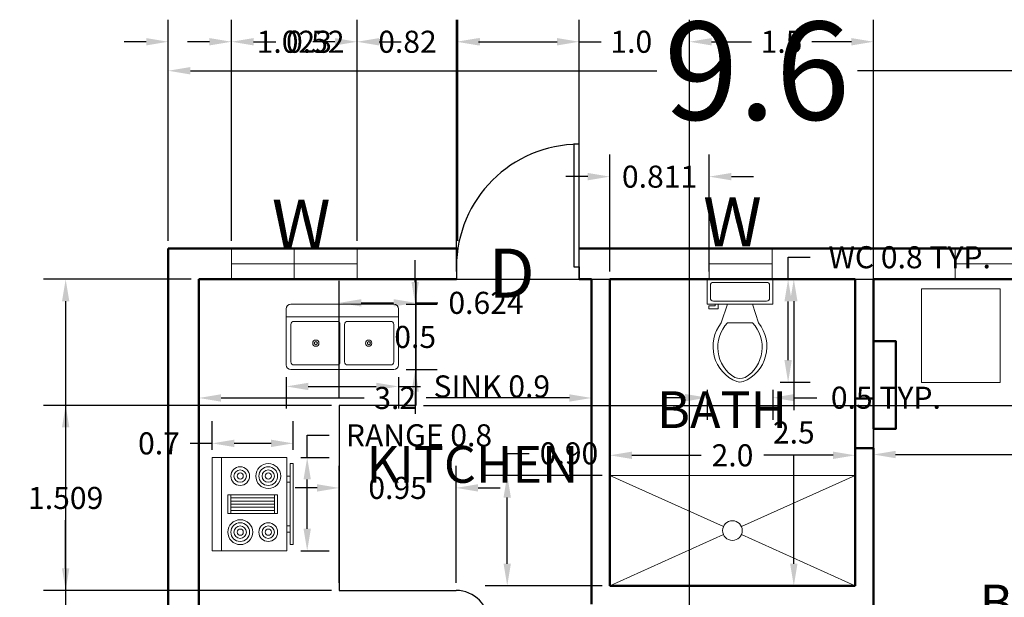
# Model space of a CAD drawing. Units: metres. Extents: x 3.9 to 21.3, y 24.8 to 56.5.
# Tile 5 of 6: x 4.9 to 13, y 36.1 to 40.8. Entities that reach past the tile are written whole.
import ezdxf

# ---------------------------------------------------------------- set-up
doc = ezdxf.new("R2010")
doc.units = ezdxf.units.M
doc.header["$MEASUREMENT"] = 0
for name, color, linetype, lineweight in [('A-AREA-IDEN', 3, 'Continuous', 25), ('A-EQPM', 6, 'Continuous', 18), ('A-FLOR-CASE', 8, 'Continuous', 25), ('A-FLOR-FIXT', 9, 'Continuous', 18), ('DIMENSIONS', 2, 'Continuous', 18), ('DOOR', 5, 'Continuous', 25), ('FURNITURE', 6, 'Continuous', 18), ('TEXT', 3, 'Continuous', 18), ('WALL', 1, 'Continuous', 50), ('WINDOW', 4, 'Continuous', 18)]:
    doc.layers.add(name, color=color, linetype=linetype, lineweight=lineweight)
doc.styles.get("Standard").update_dxf_attribs({"font": 'arial.ttf'})
doc.dimstyles.get("Standard").update_dxf_attribs({"dimtxt": 0.18, "dimasz": 0.18, "dimexe": 0.18, "dimexo": 0.0625, "dimgap": 0.09, "dimtad": 0, "dimtih": 1, "dimtoh": 1, "dimdec": 1, "dimzin": 0, "dimdsep": 46, "dimtxsty": 'Standard', "dimcen": 0.09, "dimadec": 0, "dimazin": 0, "dimtfac": 1, "dimtdec": 1, "dimtofl": 0, "dimtmove": 0, "dimatfit": 3, "dimfxl": 1, "dimtolj": 1, "dimtzin": 0, "dimarcsym": 0})

# ---------------------------------------------------------------- blocks, each defined once
blk = doc.blocks.new('*U3')
for p, q in [((0, 0), (0, -100)), ((-1000, 0), (-1000, -100))]:
    blk.add_line(p, q)
blk.add_lwpolyline([(0, 0), (0, 1000), (-43.75, 1000), (-43.75, 0)], close=True)
blk.add_arc((0, 0), 1000, 90, 180)
blk = doc.blocks.new('Range-Oven - 30 in top')
for p, q in [((0, -3), (30, -3)), ((12, -6), (18, -6)), ((13, -20), (13, -6)), ((14, -6), (14, -20)), ((15, -20), (15, -6)), ((16, -6), (16, -20)), ((17, -20), (17, -6)), ((18, -20), (12, -20)), ((6, -24), (6, -25)), ((8, -25), (8, -24)), ((22, -25), (22, -24)), ((24, -24), (24, -25))]:
    blk.add_line(p, q)
for points in [[(0, -24), (0, 0), (30, 0), (30, -24)], [(12, -21), (12, -5), (18, -5), (18, -21)], [(2, -26), (2, -25), (28, -25), (28, -26)]]:
    blk.add_lwpolyline(points, close=True)
for centre, radius in [((6, -9), 4), ((6, -9), 3), ((24, -9), 3), ((6, -9), 2), ((6, -9), 1), ((24, -9), 2), ((24, -9), 1), ((6, -18), 3), ((24, -18), 4), ((24, -18), 3), ((6, -18), 2), ((6, -18), 1), ((24, -18), 2), ((24, -18), 1)]:
    blk.add_circle(centre, radius)
blk = doc.blocks.new('Sink-double - 36 in top')
for p, q in [((-18, -4), (18, -4)), ((-0.75, -18.5), (-0.75, -6.5)), ((0.75, -6.5), (0.75, -18.5))]:
    blk.add_line(p, q)
for points in [[(-16.5, 0), (16.5, 0)], [(-18, -19.5), (-18, -1.5)], [(18, -1.5), (18, -19.5)], [(-15.5, -5.5), (-1.75, -5.5)], [(1.75, -5.5), (15.5, -5.5)], [(-16.5, -18.5), (-16.5, -6.5)], [(16.5, -6.5), (16.5, -18.5)], [(16.5, -21), (-16.5, -21)], [(-1.75, -19.5), (-15.5, -19.5)], [(15.5, -19.5), (1.75, -19.5)]]:
    blk.add_lwpolyline(points)
for centre, radius in [((-8.5, -12.5), 1), ((-8.5, -12.5), 0.5), ((8.5, -12.5), 1), ((8.5, -12.5), 0.5)]:
    blk.add_circle(centre, radius)
for centre, radius, start, end in [((-16.5, -1.5), 1.5, 90, 180), ((16.5, -1.5), 1.5, 0, 90), ((-15.5, -6.5), 1, 90, 180), ((-1.75, -6.5), 1, 0, 90), ((1.75, -6.5), 1, 90, 180), ((15.5, -6.5), 1, 0, 90), ((-15.5, -18.5), 1, 180, 270), ((-1.75, -18.5), 1, 270, 0), ((1.75, -18.5), 1, 180, 270), ((15.5, -18.5), 1, 270, 0), ((-16.5, -19.5), 1.5, 180, 270), ((16.5, -19.5), 1.5, 270, 0)]:
    blk.add_arc(centre, radius, start, end)
blk = doc.blocks.new('Toilet - top')
for p, q in [((9.5, -6), (9.5, -2)), ((-10, -8.5), (-8, -8.5)), ((-10, -9.5), (-10, -8.5)), ((-8, -8.5), (-8, -8)), ((-7, -8), (-7, -9.5)), ((-4, -8), (-6, -14)), ((4, -8), (6, -14)), ((-7, -9.5), (-10, -9.5)), ((4, -14), (-4, -14))]:
    blk.add_line(p, q)
blk.add_lwpolyline([(10.5, -8), (10.5, 0), (-10.5, 0), (-10.5, -8)], close=True)
for points in [[(-9.5, -2), (-9.5, -6)], [(8.5, -1), (-8.5, -1)], [(-8.5, -7), (8.5, -7)]]:
    blk.add_lwpolyline(points)
for centre, radius, start, end in [((-8.62, -1.88), 0.884, 81.8699, 188.1301), ((8.62, -1.88), 0.884, 351.8699, 98.1301), ((-8.62, -6.12), 0.884, 171.8699, 278.1301), ((8.62, -6.12), 0.884, 261.8699, 8.1301), ((3.52, -21.58), 12.17, 141.4691, 247.9714), ((4.2, -21.82), 11.33, 136.3677, 238.9468), ((-3.52, -21.58), 12.17, 292.0284, 38.5307), ((-4.2, -21.82), 11.33, 301.053, 43.6321), ((0, -27.88), 4, 245.7318, 294.2682), ((0, -29), 4, 254.8605, 285.1395)]:
    blk.add_arc(centre, radius, start, end)
blk = doc.blocks.new('*D22')
at = {"layer": 'Defpoints', "color": 0, "transparency": 16777216}
for p in [(15.7571, 40.3451), (6.1571, 38.8951), (15.7571, 38.8951)]:
    blk.add_point(p, dxfattribs=at)
at = {"layer": 'DIMENSIONS', "color": 0, "lineweight": -2, "transparency": 16777216}
for p, q in [((6.1571, 38.9576), (6.1571, 40.5251)), ((15.7571, 38.9576), (15.7571, 40.5251)), ((6.3371, 40.3451), (10.1392, 40.3451)), ((15.5771, 40.3451), (11.7751, 40.3451))]:
    blk.add_line(p, q, dxfattribs=at)
at = {"layer": 'DIMENSIONS', "color": 0, "transparency": 16777216}
for points in [[(6.3371, 40.3751), (6.3371, 40.3151), (6.1571, 40.3451)], [(15.5771, 40.3751), (15.5771, 40.3151), (15.7571, 40.3451)]]:
    blk.add_solid(points, dxfattribs=at)
at = {"layer": 'DIMENSIONS', "color": 0, "transparency": 16777216, "insert": (10.9571, 40.3451), "char_height": 0.18, "attachment_point": 5}
blk.add_mtext('\\A1;{\\H4.44444x;9.6}', dxfattribs=at)
blk = doc.blocks.new('*D23')
at = {"layer": 'Defpoints', "color": 0, "transparency": 16777216}
for p in [(6.4071, 37.6766), (9.6071, 37.6766), (9.6071, 37.6766)]:
    blk.add_point(p, dxfattribs=at)
at = {"layer": 'DIMENSIONS', "color": 0, "lineweight": -2, "transparency": 16777216}
for p, q in [((6.4071, 37.7391), (6.4071, 37.8566)), ((9.6071, 37.7391), (9.6071, 37.8566)), ((6.5871, 37.6766), (7.7543, 37.6766)), ((9.4271, 37.6766), (8.26, 37.6766))]:
    blk.add_line(p, q, dxfattribs=at)
at = {"layer": 'DIMENSIONS', "color": 0, "transparency": 16777216}
for points in [[(6.5871, 37.7066), (6.5871, 37.6466), (6.4071, 37.6766)], [(9.4271, 37.7066), (9.4271, 37.6466), (9.6071, 37.6766)]]:
    blk.add_solid(points, dxfattribs=at)
at = {"layer": 'DIMENSIONS', "color": 0, "transparency": 16777216, "insert": (8.0071, 37.6766), "char_height": 0.18, "attachment_point": 5}
blk.add_mtext('\\A1;3.2', dxfattribs=at)
blk = doc.blocks.new('*D24')
at = {"layer": 'Defpoints', "color": 0, "transparency": 16777216}
for p in [(9.7571, 37.2089), (11.7571, 37.2089), (11.7571, 37.2089)]:
    blk.add_point(p, dxfattribs=at)
at = {"layer": 'DIMENSIONS', "color": 0, "lineweight": -2, "transparency": 16777216}
for p, q in [((9.7571, 37.2714), (9.7571, 37.3889)), ((11.7571, 37.2714), (11.7571, 37.3889)), ((9.9371, 37.2089), (10.502, 37.2089)), ((11.5771, 37.2089), (11.0122, 37.2089))]:
    blk.add_line(p, q, dxfattribs=at)
at = {"layer": 'DIMENSIONS', "color": 0, "transparency": 16777216}
for points in [[(9.9371, 37.2389), (9.9371, 37.1789), (9.7571, 37.2089)], [(11.5771, 37.2389), (11.5771, 37.1789), (11.7571, 37.2089)]]:
    blk.add_solid(points, dxfattribs=at)
at = {"layer": 'DIMENSIONS', "color": 0, "transparency": 16777216, "insert": (10.7571, 37.2089), "char_height": 0.18, "attachment_point": 5}
blk.add_mtext('\\A1;2.0', dxfattribs=at)
blk = doc.blocks.new('*D25')
at = {"layer": 'Defpoints', "color": 0, "transparency": 16777216}
for p in [(11.9071, 37.772), (15.5071, 37.772), (15.5071, 37.2152)]:
    blk.add_point(p, dxfattribs=at)
at = {"layer": 'DIMENSIONS', "color": 0, "lineweight": -2, "transparency": 16777216}
for p, q in [((11.9071, 37.7095), (11.9071, 37.0352)), ((15.5071, 37.7095), (15.5071, 37.0352)), ((12.0871, 37.2152), (13.4534, 37.2152)), ((15.3271, 37.2152), (13.9609, 37.2152))]:
    blk.add_line(p, q, dxfattribs=at)
at = {"layer": 'DIMENSIONS', "color": 0, "transparency": 16777216}
for points in [[(12.0871, 37.2452), (12.0871, 37.1852), (11.9071, 37.2152)], [(15.3271, 37.2452), (15.3271, 37.1852), (15.5071, 37.2152)]]:
    blk.add_solid(points, dxfattribs=at)
at = {"layer": 'DIMENSIONS', "color": 0, "transparency": 16777216, "insert": (13.7071, 37.2152), "char_height": 0.18, "attachment_point": 5}
blk.add_mtext('\\A1;3.6', dxfattribs=at)
blk = doc.blocks.new('*D27')
at = {"layer": 'Defpoints', "color": 0, "transparency": 16777216}
for p in [(11.7571, 38.6451), (11.2571, 36.1451), (11.7571, 36.1451)]:
    blk.add_point(p, dxfattribs=at)
at = {"layer": 'DIMENSIONS', "color": 0, "lineweight": -2, "transparency": 16777216}
for p, q in [((11.6946, 38.6451), (11.0771, 38.6451)), ((11.2571, 38.4651), (11.2571, 37.577)), ((11.2571, 36.3251), (11.2571, 37.2132)), ((11.6946, 36.1451), (11.0771, 36.1451))]:
    blk.add_line(p, q, dxfattribs=at)
at = {"layer": 'DIMENSIONS', "color": 0, "transparency": 16777216}
for points in [[(11.2271, 38.4651), (11.2871, 38.4651), (11.2571, 38.6451)], [(11.2271, 36.3251), (11.2871, 36.3251), (11.2571, 36.1451)]]:
    blk.add_solid(points, dxfattribs=at)
at = {"layer": 'DIMENSIONS', "color": 0, "transparency": 16777216, "insert": (11.2571, 37.3951), "char_height": 0.18, "attachment_point": 5}
blk.add_mtext('\\A1;2.5', dxfattribs=at)
blk = doc.blocks.new('WIN-4-LIGHT-2046')
for p, q in [((0.5115, -0.125), (0, -0.125)), ((0.5115, -0.125), (1.0231, -0.125)), ((1.5346, -0.125), (1.0231, -0.125)), ((1.5346, -0.125), (2.0462, -0.125))]:
    blk.add_line(p, q)
for points in [[(0.5115, 0), (0, 0), (0, -0.25), (0.5115, -0.25)], [(0.5115, 0), (1.0231, 0), (1.0231, -0.25), (0.5115, -0.25)], [(1.5346, 0), (1.0231, 0), (1.0231, -0.25), (1.5346, -0.25)], [(1.5346, 0), (2.0462, 0), (2.0462, -0.25), (1.5346, -0.25)]]:
    blk.add_lwpolyline(points, close=True)
blk = doc.blocks.new('WIN-1-LIGHT-512')
blk.add_line((0, -0.125), (0.5115, -0.125))
blk.add_lwpolyline([(0, 0), (0.5115, 0), (0.5115, -0.25), (0, -0.25)], close=True)
blk = doc.blocks.new('*D45')
at = {"layer": 'Defpoints', "color": 0, "transparency": 16777216}
for p in [(11.0848, 38.6443), (11.2107, 38.6443), (11.0848, 37.8049)]:
    blk.add_point(p, dxfattribs=at)
at = {"layer": 'DIMENSIONS', "color": 0, "lineweight": -2, "transparency": 16777216}
for p, q in [((11.2107, 38.6443), (11.2107, 38.8243)), ((11.2107, 38.8243), (11.3907, 38.8243)), ((11.1473, 38.6443), (11.3907, 38.6443)), ((11.2107, 37.9849), (11.2107, 38.4643)), ((11.1473, 37.8049), (11.3907, 37.8049))]:
    blk.add_line(p, q, dxfattribs=at)
at = {"layer": 'DIMENSIONS', "color": 0, "transparency": 16777216}
for points in [[(11.1807, 38.4643), (11.2407, 38.4643), (11.2107, 38.6443)], [(11.1807, 37.9849), (11.2407, 37.9849), (11.2107, 37.8049)]]:
    blk.add_solid(points, dxfattribs=at)
at = {"layer": 'DIMENSIONS', "color": 0, "transparency": 16777216, "insert": (12.2018, 38.8243), "char_height": 0.18, "attachment_point": 5}
blk.add_mtext('\\A1;WC 0.8 TYP.', dxfattribs=at)
blk = doc.blocks.new('*D46')
at = {"layer": 'Defpoints', "color": 0, "transparency": 16777216}
for p in [(10.5514, 37.8049), (11.0848, 37.8049), (11.0848, 37.679)]:
    blk.add_point(p, dxfattribs=at)
at = {"layer": 'DIMENSIONS', "color": 0, "lineweight": -2, "transparency": 16777216}
for p, q in [((10.5514, 37.7424), (10.5514, 37.499)), ((11.0848, 37.7424), (11.0848, 37.499)), ((10.3714, 37.679), (10.1914, 37.679)), ((11.2648, 37.679), (11.4448, 37.679))]:
    blk.add_line(p, q, dxfattribs=at)
at = {"layer": 'DIMENSIONS', "color": 0, "transparency": 16777216}
for points in [[(10.3714, 37.709), (10.3714, 37.649), (10.5514, 37.679)], [(11.2648, 37.709), (11.2648, 37.649), (11.0848, 37.679)]]:
    blk.add_solid(points, dxfattribs=at)
at = {"layer": 'DIMENSIONS', "color": 0, "transparency": 16777216, "insert": (12.0078, 37.679), "char_height": 0.18, "attachment_point": 5}
blk.add_mtext('\\A1;0.5 TYP.', dxfattribs=at)
blk = doc.blocks.new('*D53')
at = {"layer": 'Defpoints', "color": 0, "transparency": 16777216}
for p in [(7.1755, 37.1919), (7.2898, 37.1919), (7.1755, 36.4299)]:
    blk.add_point(p, dxfattribs=at)
at = {"layer": 'DIMENSIONS', "color": 0, "lineweight": -2, "transparency": 16777216}
for p, q in [((7.2898, 37.1919), (7.2898, 37.3719)), ((7.2898, 37.3719), (7.4698, 37.3719)), ((7.238, 37.1919), (7.4698, 37.1919)), ((7.2898, 36.6099), (7.2898, 37.0119)), ((7.238, 36.4299), (7.4698, 36.4299))]:
    blk.add_line(p, q, dxfattribs=at)
at = {"layer": 'DIMENSIONS', "color": 0, "transparency": 16777216}
for points in [[(7.2598, 37.0119), (7.3198, 37.0119), (7.2898, 37.1919)], [(7.2598, 36.6099), (7.3198, 36.6099), (7.2898, 36.4299)]]:
    blk.add_solid(points, dxfattribs=at)
at = {"layer": 'DIMENSIONS', "color": 0, "transparency": 16777216, "insert": (8.2012, 37.3719), "char_height": 0.18, "attachment_point": 5}
blk.add_mtext('\\A1;RANGE 0.8', dxfattribs=at)
blk = doc.blocks.new('*D54')
at = {"layer": 'Defpoints', "color": 0, "transparency": 16777216}
for p in [(6.5151, 37.3062), (6.5151, 37.1919), (7.1755, 37.1919)]:
    blk.add_point(p, dxfattribs=at)
at = {"layer": 'DIMENSIONS', "color": 0, "lineweight": -2, "transparency": 16777216}
for p, q in [((6.5151, 37.2544), (6.5151, 37.4862)), ((7.1755, 37.2544), (7.1755, 37.4862)), ((6.5151, 37.3062), (6.3351, 37.3062)), ((6.9955, 37.3062), (6.6951, 37.3062))]:
    blk.add_line(p, q, dxfattribs=at)
at = {"layer": 'DIMENSIONS', "color": 0, "transparency": 16777216}
for points in [[(6.6951, 37.3362), (6.6951, 37.2762), (6.5151, 37.3062)], [(6.9955, 37.3362), (6.9955, 37.2762), (7.1755, 37.3062)]]:
    blk.add_solid(points, dxfattribs=at)
at = {"layer": 'DIMENSIONS', "color": 0, "transparency": 16777216, "insert": (6.0812, 37.3062), "char_height": 0.18, "attachment_point": 5}
blk.add_mtext('\\A1;0.7', dxfattribs=at)
blk = doc.blocks.new('*D55')
at = {"layer": 'Defpoints', "color": 0, "transparency": 16777216}
for p in [(7.1188, 37.9077), (8.0332, 37.9077), (8.0332, 37.7706)]:
    blk.add_point(p, dxfattribs=at)
at = {"layer": 'DIMENSIONS', "color": 0, "lineweight": -2, "transparency": 16777216}
for p, q in [((7.1188, 37.8452), (7.1188, 37.5906)), ((8.0332, 37.8452), (8.0332, 37.5906)), ((7.2988, 37.7706), (7.8532, 37.7706)), ((8.0332, 37.7706), (8.2132, 37.7706))]:
    blk.add_line(p, q, dxfattribs=at)
at = {"layer": 'DIMENSIONS', "color": 0, "transparency": 16777216}
for points in [[(7.2988, 37.8006), (7.2988, 37.7406), (7.1188, 37.7706)], [(7.8532, 37.8006), (7.8532, 37.7406), (8.0332, 37.7706)]]:
    blk.add_solid(points, dxfattribs=at)
at = {"layer": 'DIMENSIONS', "color": 0, "transparency": 16777216, "insert": (8.7952, 37.7706), "char_height": 0.18, "attachment_point": 5}
blk.add_mtext('\\A1;SINK 0.9', dxfattribs=at)
blk = doc.blocks.new('*D56')
at = {"layer": 'Defpoints', "color": 0, "transparency": 16777216}
for p in [(8.0332, 38.4411), (8.1703, 38.4411), (8.0332, 37.9077)]:
    blk.add_point(p, dxfattribs=at)
at = {"layer": 'DIMENSIONS', "color": 0, "lineweight": -2, "transparency": 16777216}
for p, q in [((8.1703, 38.6211), (8.1703, 38.8011)), ((8.0957, 38.4411), (8.3503, 38.4411)), ((8.0957, 37.9077), (8.3503, 37.9077)), ((8.1703, 37.7277), (8.1703, 37.5477))]:
    blk.add_line(p, q, dxfattribs=at)
at = {"layer": 'DIMENSIONS', "color": 0, "transparency": 16777216}
for points in [[(8.1403, 38.6211), (8.2003, 38.6211), (8.1703, 38.4411)], [(8.1403, 37.7277), (8.2003, 37.7277), (8.1703, 37.9077)]]:
    blk.add_solid(points, dxfattribs=at)
at = {"layer": 'DIMENSIONS', "color": 0, "transparency": 16777216, "insert": (8.1703, 38.1744), "char_height": 0.18, "attachment_point": 5}
blk.add_mtext('\\A1;0.5', dxfattribs=at)
blk = doc.blocks.new('*D76')
at = {"layer": 'Defpoints', "color": 0, "transparency": 16777216}
for p in [(6.4071, 38.6451), (5.3206, 28.2303), (6.4071, 28.2303)]:
    blk.add_point(p, dxfattribs=at)
at = {"layer": 'DIMENSIONS', "color": 0, "lineweight": -2, "transparency": 16777216}
for p, q in [((6.3446, 38.6451), (5.1406, 38.6451)), ((5.3206, 38.4651), (5.3206, 33.6196)), ((5.3206, 28.4103), (5.3206, 33.2558)), ((6.3446, 28.2303), (5.1406, 28.2303))]:
    blk.add_line(p, q, dxfattribs=at)
at = {"layer": 'DIMENSIONS', "color": 0, "transparency": 16777216}
for points in [[(5.2906, 38.4651), (5.3506, 38.4651), (5.3206, 38.6451)], [(5.2906, 28.4103), (5.3506, 28.4103), (5.3206, 28.2303)]]:
    blk.add_solid(points, dxfattribs=at)
at = {"layer": 'DIMENSIONS', "color": 0, "transparency": 16777216, "insert": (5.3206, 33.4377), "char_height": 0.18, "attachment_point": 5}
blk.add_mtext('\\A1;10.415', dxfattribs=at)
blk = doc.blocks.new('*D77')
at = {"layer": 'Defpoints', "color": 0, "transparency": 16777216}
for p in [(11.9071, 40.5816), (10.4071, 33.623), (11.9071, 33.623)]:
    blk.add_point(p, dxfattribs=at)
at = {"layer": 'DIMENSIONS', "color": 0, "lineweight": -2, "transparency": 16777216}
for p, q in [((10.4071, 33.6855), (10.4071, 40.7616)), ((11.9071, 33.6855), (11.9071, 40.7616)), ((10.5871, 40.5816), (10.9111, 40.5816)), ((11.7271, 40.5816), (11.4032, 40.5816))]:
    blk.add_line(p, q, dxfattribs=at)
at = {"layer": 'DIMENSIONS', "color": 0, "transparency": 16777216}
for points in [[(10.5871, 40.6116), (10.5871, 40.5516), (10.4071, 40.5816)], [(11.7271, 40.6116), (11.7271, 40.5516), (11.9071, 40.5816)]]:
    blk.add_solid(points, dxfattribs=at)
at = {"layer": 'DIMENSIONS', "color": 0, "transparency": 16777216, "insert": (11.1571, 40.5816), "char_height": 0.18, "attachment_point": 5}
blk.add_mtext('\\A1;1.5', dxfattribs=at)
blk = doc.blocks.new('*D81')
at = {"layer": 'Defpoints', "color": 0, "transparency": 16777216}
for p in [(6.6728, 40.5816), (6.1571, 38.8951), (6.6728, 38.8951)]:
    blk.add_point(p, dxfattribs=at)
at = {"layer": 'DIMENSIONS', "color": 0, "lineweight": -2, "transparency": 16777216}
for p, q in [((6.1571, 38.9576), (6.1571, 40.7616)), ((6.6728, 38.9576), (6.6728, 40.7616)), ((5.9771, 40.5816), (5.7971, 40.5816)), ((6.8528, 40.5816), (7.0328, 40.5816))]:
    blk.add_line(p, q, dxfattribs=at)
at = {"layer": 'DIMENSIONS', "color": 0, "transparency": 16777216}
for points in [[(5.9771, 40.6116), (5.9771, 40.5516), (6.1571, 40.5816)], [(6.8528, 40.6116), (6.8528, 40.5516), (6.6728, 40.5816)]]:
    blk.add_solid(points, dxfattribs=at)
at = {"layer": 'DIMENSIONS', "color": 0, "transparency": 16777216, "insert": (7.3557, 40.5816), "char_height": 0.18, "attachment_point": 5}
blk.add_mtext('\\A1;0.52', dxfattribs=at)
blk = doc.blocks.new('*D82')
at = {"layer": 'Defpoints', "color": 0, "transparency": 16777216}
for p in [(7.6959, 40.5816), (6.6728, 38.8951), (7.6959, 38.8951)]:
    blk.add_point(p, dxfattribs=at)
at = {"layer": 'DIMENSIONS', "color": 0, "lineweight": -2, "transparency": 16777216}
for p, q in [((6.6728, 38.9576), (6.6728, 40.7616)), ((7.6959, 38.9576), (7.6959, 40.7616)), ((6.4928, 40.5816), (6.3128, 40.5816)), ((7.8759, 40.5816), (8.0559, 40.5816))]:
    blk.add_line(p, q, dxfattribs=at)
at = {"layer": 'DIMENSIONS', "color": 0, "transparency": 16777216}
for points in [[(6.4928, 40.6116), (6.4928, 40.5516), (6.6728, 40.5816)], [(7.8759, 40.6116), (7.8759, 40.5516), (7.6959, 40.5816)]]:
    blk.add_solid(points, dxfattribs=at)
at = {"layer": 'DIMENSIONS', "color": 0, "transparency": 16777216, "insert": (7.1843, 40.5816), "char_height": 0.18, "attachment_point": 5}
blk.add_mtext('\\A1;1.023', dxfattribs=at)
blk = doc.blocks.new('*D83')
at = {"layer": 'Defpoints', "color": 0, "transparency": 16777216}
for p in [(8.5184, 40.5816), (7.6959, 38.8951), (8.5184, 38.8951)]:
    blk.add_point(p, dxfattribs=at)
at = {"layer": 'DIMENSIONS', "color": 0, "lineweight": -2, "transparency": 16777216}
for p, q in [((7.6959, 38.9576), (7.6959, 40.7616)), ((8.5184, 38.9576), (8.5184, 40.7616)), ((7.5159, 40.5816), (7.3359, 40.5816)), ((8.6984, 40.5816), (8.8784, 40.5816))]:
    blk.add_line(p, q, dxfattribs=at)
at = {"layer": 'DIMENSIONS', "color": 0, "transparency": 16777216}
for points in [[(7.5159, 40.6116), (7.5159, 40.5516), (7.6959, 40.5816)], [(8.6984, 40.6116), (8.6984, 40.5516), (8.5184, 40.5816)]]:
    blk.add_solid(points, dxfattribs=at)
at = {"layer": 'DIMENSIONS', "color": 0, "transparency": 16777216, "insert": (8.1072, 40.5816), "char_height": 0.18, "attachment_point": 5}
blk.add_mtext('\\A1;0.82', dxfattribs=at)
blk = doc.blocks.new('*D84')
at = {"layer": 'Defpoints', "color": 0, "transparency": 16777216}
for p in [(9.5071, 40.5816), (8.5071, 38.6451), (9.5071, 38.6451)]:
    blk.add_point(p, dxfattribs=at)
at = {"layer": 'DIMENSIONS', "color": 0, "lineweight": -2, "transparency": 16777216}
for p, q in [((8.5071, 38.7076), (8.5071, 40.7616)), ((9.5071, 38.7076), (9.5071, 40.7616)), ((8.6871, 40.5816), (9.3271, 40.5816)), ((9.5071, 40.5816), (9.6871, 40.5816))]:
    blk.add_line(p, q, dxfattribs=at)
at = {"layer": 'DIMENSIONS', "color": 0, "transparency": 16777216}
for points in [[(8.6871, 40.6116), (8.6871, 40.5516), (8.5071, 40.5816)], [(9.3271, 40.6116), (9.3271, 40.5516), (9.5071, 40.5816)]]:
    blk.add_solid(points, dxfattribs=at)
at = {"layer": 'DIMENSIONS', "color": 0, "transparency": 16777216, "insert": (9.9322, 40.5816), "char_height": 0.18, "attachment_point": 5}
blk.add_mtext('\\A1;1.0', dxfattribs=at)
blk = doc.blocks.new('*D85')
at = {"layer": 'Defpoints', "color": 0, "transparency": 16777216}
for p in [(10.568072, 39.481572), (9.757128, 38.645072), (10.568072, 38.645072)]:
    blk.add_point(p, dxfattribs=at)
at = {"layer": 'DIMENSIONS', "color": 0, "lineweight": -2, "transparency": 16777216}
for p, q in [((9.757128, 38.707572), (9.757128, 39.661572)), ((10.568072, 38.707572), (10.568072, 39.661572)), ((9.577128, 39.481572), (9.397128, 39.481572)), ((10.748072, 39.481572), (10.928072, 39.481572))]:
    blk.add_line(p, q, dxfattribs=at)
at = {"layer": 'DIMENSIONS', "color": 0, "transparency": 16777216}
for points in [[(9.577128, 39.511572), (9.577128, 39.451572), (9.757128, 39.481572)], [(10.748072, 39.511572), (10.748072, 39.451572), (10.568072, 39.481572)]]:
    blk.add_solid(points, dxfattribs=at)
at = {"layer": 'DIMENSIONS', "color": 0, "transparency": 16777216, "insert": (10.1626, 39.481572), "char_height": 0.18, "attachment_point": 5}
blk.add_mtext('\\A1;0.811', dxfattribs=at)
blk = doc.blocks.new('*D95')
at = {"layer": 'Defpoints', "color": 0, "transparency": 16777216}
for p in [(8.9206, 37.0447), (9.7571, 37.0447), (9.7571, 36.1451)]:
    blk.add_point(p, dxfattribs=at)
at = {"layer": 'DIMENSIONS', "color": 0, "lineweight": -2, "transparency": 16777216}
for p, q in [((8.9206, 37.0447), (8.9206, 37.2247)), ((8.9206, 37.2247), (9.1006, 37.2247)), ((9.6946, 37.0447), (8.7406, 37.0447)), ((8.9206, 36.3251), (8.9206, 36.8647)), ((9.6946, 36.1451), (8.7406, 36.1451))]:
    blk.add_line(p, q, dxfattribs=at)
at = {"layer": 'DIMENSIONS', "color": 0, "transparency": 16777216}
for points in [[(8.8906, 36.8647), (8.9506, 36.8647), (8.9206, 37.0447)], [(8.8906, 36.3251), (8.9506, 36.3251), (8.9206, 36.1451)]]:
    blk.add_solid(points, dxfattribs=at)
at = {"layer": 'DIMENSIONS', "color": 0, "transparency": 16777216, "insert": (9.4241, 37.2247), "char_height": 0.18, "attachment_point": 5}
blk.add_mtext('\\A1;0.90', dxfattribs=at)
blk = doc.blocks.new('*D97')
at = {"layer": 'Defpoints', "color": 0, "transparency": 16777216}
for p in [(8.503283, 36.94312), (7.550403, 36.10662), (8.503283, 36.10662)]:
    blk.add_point(p, dxfattribs=at)
at = {"layer": 'DIMENSIONS', "color": 0, "lineweight": -2, "transparency": 16777216}
for p, q in [((7.550403, 36.16912), (7.550403, 37.12312)), ((8.503283, 36.16912), (8.503283, 37.12312)), ((7.370403, 36.94312), (7.190403, 36.94312)), ((8.683283, 36.94312), (8.863283, 36.94312))]:
    blk.add_line(p, q, dxfattribs=at)
at = {"layer": 'DIMENSIONS', "color": 0, "transparency": 16777216}
for points in [[(7.370403, 36.97312), (7.370403, 36.91312), (7.550403, 36.94312)], [(8.683283, 36.97312), (8.683283, 36.91312), (8.503283, 36.94312)]]:
    blk.add_solid(points, dxfattribs=at)
at = {"layer": 'DIMENSIONS', "color": 0, "transparency": 16777216, "insert": (8.026843, 36.94312), "char_height": 0.18, "attachment_point": 5}
blk.add_mtext('\\A1;0.95', dxfattribs=at)
blk = doc.blocks.new('*D98')
at = {"layer": 'Defpoints', "color": 0, "transparency": 16777216}
for p in [(5.3206, 37.6158), (7.5504, 37.6158), (7.5504, 36.1066)]:
    blk.add_point(p, dxfattribs=at)
at = {"layer": 'DIMENSIONS', "color": 0, "lineweight": -2, "transparency": 16777216}
for p, q in [((7.4879, 37.6158), (5.1406, 37.6158)), ((5.3206, 37.4358), (5.3206, 37.0431)), ((5.3206, 36.2866), (5.3206, 36.6793)), ((7.4879, 36.1066), (5.1406, 36.1066))]:
    blk.add_line(p, q, dxfattribs=at)
at = {"layer": 'DIMENSIONS', "color": 0, "transparency": 16777216}
for points in [[(5.2906, 37.4358), (5.3506, 37.4358), (5.3206, 37.6158)], [(5.2906, 36.2866), (5.3506, 36.2866), (5.3206, 36.1066)]]:
    blk.add_solid(points, dxfattribs=at)
at = {"layer": 'DIMENSIONS', "color": 0, "transparency": 16777216, "insert": (5.3206, 36.8612), "char_height": 0.18, "attachment_point": 5}
blk.add_mtext('\\A1;1.509', dxfattribs=at)
blk = doc.blocks.new('*D99')
at = {"layer": 'Defpoints', "color": 0, "transparency": 16777216}
for p in [(8.1743, 38.4523), (7.5504, 37.6158), (8.1743, 37.6158)]:
    blk.add_point(p, dxfattribs=at)
at = {"layer": 'DIMENSIONS', "color": 0, "lineweight": -2, "transparency": 16777216}
for p, q in [((7.5504, 37.6783), (7.5504, 38.6323)), ((8.1743, 37.6783), (8.1743, 38.6323)), ((7.7304, 38.4523), (7.9943, 38.4523)), ((8.1743, 38.4523), (8.3543, 38.4523))]:
    blk.add_line(p, q, dxfattribs=at)
at = {"layer": 'DIMENSIONS', "color": 0, "transparency": 16777216}
for points in [[(7.7304, 38.4823), (7.7304, 38.4223), (7.5504, 38.4523)], [(7.9943, 38.4823), (7.9943, 38.4223), (8.1743, 38.4523)]]:
    blk.add_solid(points, dxfattribs=at)
at = {"layer": 'DIMENSIONS', "color": 0, "transparency": 16777216, "insert": (8.7477, 38.4523), "char_height": 0.18, "attachment_point": 5}
blk.add_mtext('\\A1;0.624', dxfattribs=at)
blk = doc.blocks.new('*D100')
at = {"layer": 'Defpoints', "color": 0, "transparency": 16777216}
for p in [(8.1743, 38.6451), (16.5936, 38.6451), (8.1743, 37.6158)]:
    blk.add_point(p, dxfattribs=at)
at = {"layer": 'DIMENSIONS', "color": 0, "lineweight": -2, "transparency": 16777216}
for p, q in [((8.2368, 38.6451), (16.7736, 38.6451)), ((16.5936, 38.4651), (16.5936, 38.3124)), ((16.5936, 37.7958), (16.5936, 37.9485)), ((8.2368, 37.6158), (16.7736, 37.6158))]:
    blk.add_line(p, q, dxfattribs=at)
at = {"layer": 'DIMENSIONS', "color": 0, "transparency": 16777216}
for points in [[(16.5636, 38.4651), (16.6236, 38.4651), (16.5936, 38.6451)], [(16.5636, 37.7958), (16.6236, 37.7958), (16.5936, 37.6158)]]:
    blk.add_solid(points, dxfattribs=at)
at = {"layer": 'DIMENSIONS', "color": 0, "transparency": 16777216, "insert": (16.5936, 38.1304), "char_height": 0.18, "attachment_point": 5}
blk.add_mtext('\\A1;1.03', dxfattribs=at)

msp = doc.modelspace()

# ---------------------------------------------------------------- linework, layer by layer
at = {"layer": 'A-FLOR-CASE'}
for p, q in [((8.1743, 38.6451), (8.1743, 37.6158)), ((8.1743, 37.6158), (7.5504, 37.6158)), ((7.5504, 37.6158), (7.5504, 36.1066)), ((7.5504, 36.1066), (8.5033, 36.1066))]:
    msp.add_line(p, q, dxfattribs=at)
msp.add_arc((8.5033, 35.8376), 0.269, 270, 90, dxfattribs=at)
at = {"layer": 'A-FLOR-FIXT'}
for p, q in [((9.7571, 37.0447), (11.7571, 37.0447)), ((9.7571, 37.0447), (10.684, 36.6278)), ((11.7571, 37.0447), (10.8302, 36.6278)), ((10.684, 36.562), (9.7571, 36.1451)), ((10.8302, 36.562), (11.7571, 36.1451))]:
    msp.add_line(p, q, dxfattribs=at)
msp.add_circle((10.7571, 36.5949), 0.0802, dxfattribs=at)
at = {"layer": 'DOOR'}
msp.add_line((9.5071, 38.6451), (9.5071, 38.8951), dxfattribs=at)
at = {"layer": 'FURNITURE'}
msp.add_lwpolyline([(12.9409, 38.5678), (12.2973, 38.5678), (12.2973, 37.8025), (12.9409, 37.8025)], close=True, dxfattribs=at)
at = {"layer": 'WALL'}
for p, q in [((6.1571, 38.8951), (8.5184, 38.8951)), ((6.1571, 25.8451), (6.1571, 38.8951)), ((9.5071, 38.8951), (15.7571, 38.8951)), ((6.4071, 38.6451), (8.5071, 38.6451)), ((6.4071, 28.2303), (6.4071, 38.6451)), ((9.5071, 38.6451), (9.6071, 38.6451)), ((9.6071, 35.9951), (9.6071, 38.6451)), ((9.7571, 38.6451), (11.7571, 38.6451)), ((9.7571, 36.1451), (9.7571, 38.6451)), ((11.7571, 36.1451), (11.7571, 38.6451)), ((11.9071, 38.6451), (15.5071, 38.6451)), ((11.9071, 37.4258), (11.9071, 38.6451)), ((11.7571, 37.6716), (11.9071, 37.6716)), ((11.7571, 37.2672), (11.9071, 37.2672)), ((11.9071, 35.0451), (11.9071, 37.2672)), ((9.7571, 36.1451), (11.7571, 36.1451))]:
    msp.add_line(p, q, dxfattribs=at)
msp.add_lwpolyline([(11.9071, 37.6716), (11.9071, 38.1394), (12.0895, 38.1394), (12.0895, 37.4258), (11.9071, 37.4258)], dxfattribs=at)
at = {"layer": 'WINDOW'}
for p in [(6.6728, 38.7701), (7.6959, 38.7701)]:
    msp.add_line(p, (7.1843, 38.7701), dxfattribs=at)
for points in [[(6.6728, 38.8951), (7.1843, 38.8951), (7.1843, 38.6451), (6.6728, 38.6451)], [(7.6959, 38.8951), (7.1843, 38.8951), (7.1843, 38.6451), (7.6959, 38.6451)]]:
    msp.add_lwpolyline(points, close=True, dxfattribs=at)

# ---------------------------------------------------------------- block references
at = {"layer": 'A-EQPM', "xscale": 0.0254, "yscale": 0.0254, "zscale": 0.0254, "rotation": 90}
msp.add_blockref('Range-Oven - 30 in top', (6.5151, 36.4299), dxfattribs=at)
at = {"layer": 'A-FLOR-FIXT', "xscale": 0.0254, "yscale": 0.0254, "zscale": 0.0254}
for name, p in [('Toilet - top', (10.8181, 38.6443)), ('Sink-double - 36 in top', (7.576, 38.4411))]:
    msp.add_blockref(name, p, dxfattribs=at)
at = {"layer": 'DOOR', "xscale": 0.001, "yscale": 0.001, "zscale": 0.001}
msp.add_blockref('*U3', (9.5071, 38.7451), dxfattribs=at)
at = {"layer": 'WINDOW'}
for name, p in [('WIN-1-LIGHT-512', (10.5681, 38.8951)), ('WIN-4-LIGHT-2046', (12.5738, 38.8951))]:
    msp.add_blockref(name, p, dxfattribs=at)

# ---------------------------------------------------------------- texts
at = {"layer": 'A-AREA-IDEN', "char_height": 0.3, "attachment_point": 1}
for s, width, insert in [('BATH', 1.45972, (10.142, 37.7313)), ('KITCHEN', 0.762737, (7.7749, 37.2847)), ('BEDROOM 1', 1.45972, (12.7722, 36.1551))]:
    msp.add_mtext_dynamic_manual_height_columns(s, width=width, gutter_width=1, heights=[0], dxfattribs=dict(at, insert=insert))
at = {"layer": 'TEXT', "char_height": 0.4, "attachment_point": 1}
for s, insert in [('W', (7.0016, 39.2951)), ('W', (10.5174, 39.3123)), ('D', (8.7691, 38.8951))]:
    msp.add_mtext_dynamic_manual_height_columns(s, width=0.69425, gutter_width=1, heights=[0], dxfattribs=dict(at, insert=insert))

# ---------------------------------------------------------------- dimensions: what is measured, and where the dimension line sits
at = {"layer": 'DIMENSIONS'}
for base, p1, p2, override, picture, middle in [((6.6728, 40.5816), (6.1571, 38.8951), (6.6728, 38.8951), {"dimdec": 2, "dimlfac": 1, "dimrnd": 0, "dimzin": 0, "dimdsep": 46, "dimlunit": 2}, '*D81', (7.3557, 40.5816)), ((7.6959, 40.5816), (6.6728, 38.8951), (7.6959, 38.8951), {"dimdec": 3, "dimlfac": 1, "dimrnd": 0, "dimzin": 0, "dimdsep": 46, "dimlunit": 2}, '*D82', (7.1843, 40.5816)), ((8.5184, 40.5816), (7.6959, 38.8951), (8.5184, 38.8951), {"dimdec": 2, "dimlfac": 1, "dimrnd": 0, "dimzin": 0, "dimdsep": 46, "dimlunit": 2}, '*D83', (8.1072, 40.5816)), ((9.5071, 40.5816), (8.5071, 38.6451), (9.5071, 38.6451), {"dimdec": 1, "dimlfac": 1, "dimrnd": 0, "dimzin": 0, "dimdsep": 46, "dimlunit": 2}, '*D84', (9.9322, 40.5816)), ((11.9071, 40.5816), (10.4071, 33.623), (11.9071, 33.623), {"dimdec": 1, "dimlfac": 1, "dimrnd": 0, "dimzin": 0, "dimdsep": 46, "dimlunit": 2}, '*D77', (11.1571, 40.5816)), ((8.1743, 38.4523), (7.5504, 37.6158), (8.1743, 37.6158), {"dimdec": 3, "dimlfac": 1, "dimrnd": 0, "dimzin": 0, "dimdsep": 46, "dimlunit": 2}, '*D99', (8.7477, 38.4523)), ((9.6071, 37.6766), (6.4071, 37.6766), (9.6071, 37.6766), {"dimclrd": 0, "dimclre": 0, "dimclrt": 0}, '*D23', (8.0071, 37.6766)), ((15.5071, 37.2152), (11.9071, 37.772), (15.5071, 37.772), {"dimclrd": 0, "dimclre": 0, "dimclrt": 0}, '*D25', (13.7071, 37.2152)), ((11.7571, 37.2089), (9.7571, 37.2089), (11.7571, 37.2089), {"dimclrd": 0, "dimclre": 0, "dimclrt": 0}, '*D24', (10.7571, 37.2089)), ((8.5033, 36.9431), (7.5504, 36.1066), (8.5033, 36.1066), {"dimdec": 2, "dimlfac": 1, "dimrnd": 0, "dimzin": 0, "dimdsep": 46, "dimlunit": 2}, '*D97', (8.0268, 36.9431))]:
    dim = msp.add_linear_dim(base=base, p1=p1, p2=p2, dimstyle='Standard', override=override, dxfattribs=at)
    dim.commit()
    dim.dimension.update_dxf_attribs({"geometry": picture, "text_midpoint": middle})
for base, p1, p2, text, override, picture, middle in [((15.7571, 40.3451), (6.1571, 38.8951), (15.7571, 38.8951), '{\\H4.44444x;<>}', {"dimclrd": 0, "dimclre": 0, "dimclrt": 0}, '*D22', (10.9571, 40.3451)), ((8.0332, 37.7706), (7.1188, 37.9077), (8.0332, 37.9077), 'SINK <>', {"dimdec": 1, "dimlfac": 1, "dimrnd": 0, "dimzin": 0, "dimdsep": 46, "dimlunit": 2}, '*D55', (8.7952, 37.7706)), ((11.0848, 37.679), (10.5514, 37.8049), (11.0848, 37.8049), '<> TYP.', {"dimdec": 1, "dimlfac": 1, "dimrnd": 0, "dimzin": 0, "dimdsep": 46, "dimlunit": 2}, '*D46', (12.0078, 37.679))]:
    dim = msp.add_linear_dim(base=base, p1=p1, p2=p2, text=text, dimstyle='Standard', override=override, dxfattribs=at)
    dim.commit()
    dim.dimension.update_dxf_attribs({"geometry": picture, "text_midpoint": middle})
for base, p1, p2, angle, override, picture, middle in [((10.5681, 39.4816), (9.7571, 38.6451), (10.5681, 38.6451), 0, {"dimdec": 3, "dimlfac": 1, "dimrnd": 0, "dimzin": 0, "dimdsep": 46, "dimlunit": 2}, '*D85', (10.1626, 39.4816)), ((8.1703, 38.4411), (8.0332, 37.9077), (8.0332, 38.4411), 90, {"dimdec": 1, "dimlfac": 1, "dimrnd": 0, "dimzin": 0, "dimdsep": 46, "dimlunit": 2}, '*D56', (8.1703, 38.1744)), ((5.3206, 28.2303), (6.4071, 38.6451), (6.4071, 28.2303), 90, {"dimdec": 3, "dimlfac": 1, "dimrnd": 0, "dimzin": 0, "dimdsep": 46, "dimlunit": 2}, '*D76', (5.3206, 33.4377)), ((16.5936, 38.6451), (8.1743, 37.6158), (8.1743, 38.6451), 90, {"dimdec": 2, "dimlfac": 1, "dimrnd": 0, "dimzin": 0, "dimdsep": 46, "dimlunit": 2}, '*D100', (16.5936, 38.1304)), ((11.2571, 36.1451), (11.7571, 38.6451), (11.7571, 36.1451), 90, {"dimclrd": 0, "dimclre": 0, "dimclrt": 0}, '*D27', (11.2571, 37.3951)), ((5.3206, 37.6158), (7.5504, 36.1066), (7.5504, 37.6158), 90, {"dimdec": 3, "dimlfac": 1, "dimrnd": 0, "dimzin": 0, "dimdsep": 46, "dimlunit": 2}, '*D98', (5.3206, 36.8612)), ((6.5151, 37.3062), (7.1755, 37.1919), (6.5151, 37.1919), 180, {"dimdec": 1, "dimlfac": 1, "dimrnd": 0, "dimzin": 0, "dimdsep": 46, "dimlunit": 2}, '*D54', (6.0812, 37.3062)), ((8.9206, 37.0447), (9.7571, 36.1451), (9.7571, 37.0447), 90, {"dimdec": 2, "dimlfac": 1, "dimrnd": 0, "dimzin": 0, "dimdsep": 46, "dimlunit": 2}, '*D95', (9.4241, 37.2247))]:
    dim = msp.add_linear_dim(base=base, p1=p1, p2=p2, angle=angle, dimstyle='Standard', override=override, dxfattribs=at)
    dim.commit()
    dim.dimension.update_dxf_attribs({"geometry": picture, "text_midpoint": middle})
for base, p1, p2, text, picture, middle in [((11.2107, 38.6443), (11.0848, 37.8049), (11.0848, 38.6443), 'WC <> TYP.', '*D45', (12.2018, 38.8243)), ((7.2898, 37.1919), (7.1755, 36.4299), (7.1755, 37.1919), 'RANGE <>', '*D53', (8.2012, 37.3719))]:
    dim = msp.add_linear_dim(base=base, p1=p1, p2=p2, angle=90, text=text, dimstyle='Standard', override={"dimdec": 1, "dimlfac": 1, "dimrnd": 0, "dimzin": 0, "dimdsep": 46, "dimlunit": 2}, dxfattribs=at)
    dim.commit()
    dim.dimension.update_dxf_attribs({"geometry": picture, "text_midpoint": middle})

doc.saveas('drawing.dxf')
